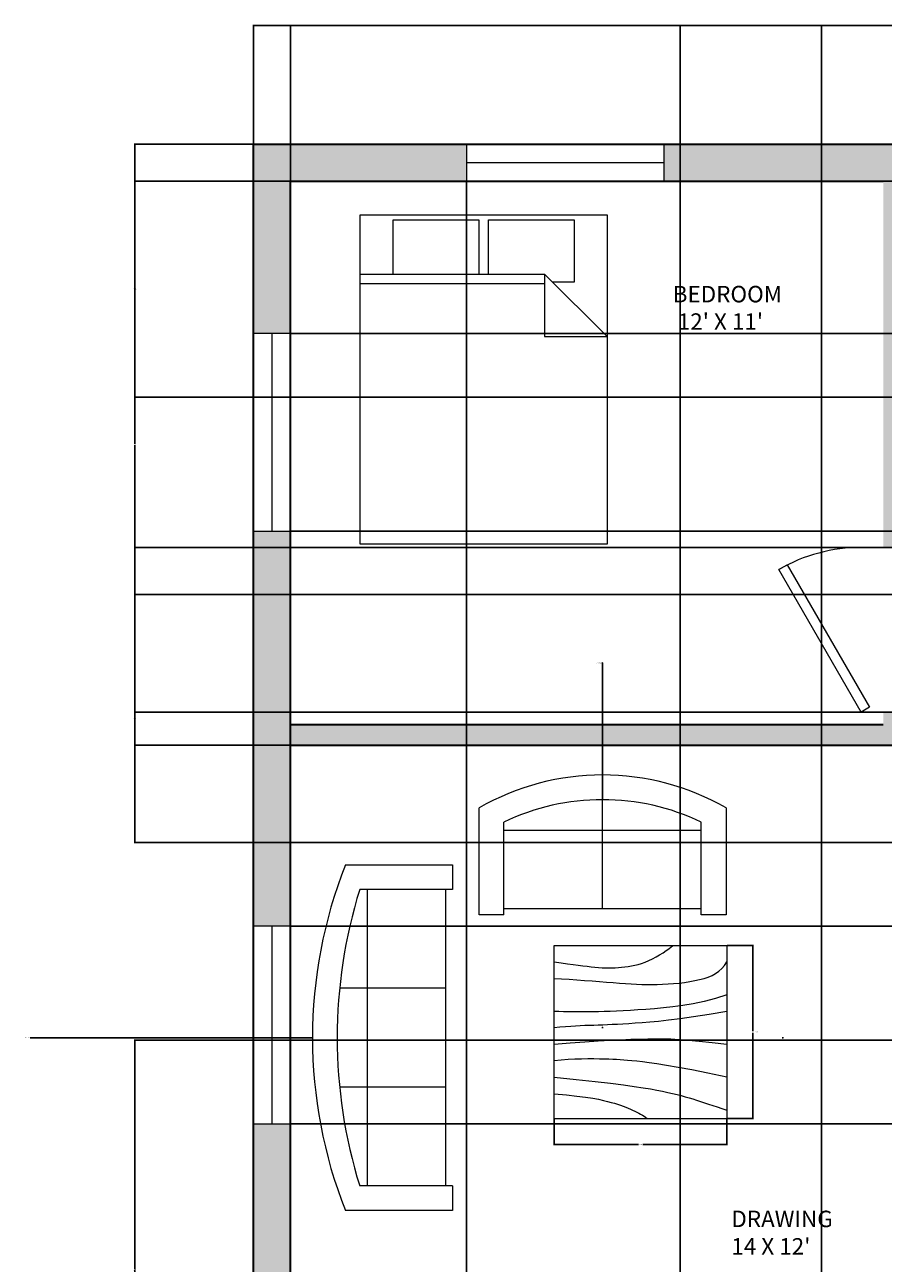
# Model space of a CAD drawing. Units: inches. Extents: x -28 to 649, y -11 to 509.
# Tile 3 of 7: x -28 to 180, y 208 to 509. Entities that reach past the tile are written whole.
import ezdxf

# ---------------------------------------------------------------- set-up
doc = ezdxf.new("R2010")
doc.units = ezdxf.units.IN
doc.header["$MEASUREMENT"] = 0
for name, color, linetype, lineweight in [('A-ANNO-DIMS', 2, 'Continuous', 18), ('A-AREA-IDEN', 18, 'Continuous', 18), ('A-WALL', 7, 'Continuous', 35), ('A-WALL-PATT', 251, 'Continuous', 13), ('doors', 40, 'Continuous', 20), ('furniture', 220, 'Continuous', 18), ('window', 30, 'Continuous', 18)]:
    doc.layers.add(name, color=color, linetype=linetype, lineweight=lineweight)
doc.styles.get("Standard").update_dxf_attribs({"font": 'arial.ttf'})
doc.dimstyles.get("Standard").update_dxf_attribs({"dimtxt": 0.18, "dimasz": 0.18, "dimexe": 0.18, "dimexo": 0.0625, "dimgap": 0.09, "dimtad": 0, "dimtih": 1, "dimtoh": 1, "dimdec": 4, "dimzin": 0, "dimdsep": 46, "dimtxsty": 'Standard', "dimcen": 0.09, "dimadec": 0, "dimazin": 0, "dimtfac": 1, "dimtdec": 4, "dimtofl": 0, "dimtmove": 0, "dimatfit": 3, "dimfxl": 1, "dimtolj": 1, "dimtzin": 0, "dimarcsym": 0})

# ---------------------------------------------------------------- blocks, each defined once
blk = doc.blocks.new('*U9')
for p, q in [((0, 0), (0, -100)), ((750, 0), (750, -100))]:
    blk.add_line(p, q)
blk.add_lwpolyline([(0, 0), (649.5, 375), (671.4, 337.1), (21.9, -37.9)], close=True)
blk.add_arc((0, 0), 750, 0, 30)
blk = doc.blocks.new('Table - Square Woodgrain 42 x 42 in.')
blk.add_line((0, -42), (42, -42))
for points in [[(0, -4), (1.704, -4.2172), (3.2358, -4.4188), (4.615, -4.604), (5.8615, -4.7721), (6.9951, -4.9224), (8.0357, -5.0541), (9.0031, -5.1667), (9.9171, -5.2594), (10.7951, -5.3316), (11.6445, -5.3836), (12.4702, -5.4157), (13.277, -5.4283), (14.0698, -5.4217), (14.8535, -5.3964), (15.6331, -5.3526), (16.4133, -5.2908), (17.1986, -5.2103), (17.9913, -5.1062), (18.793, -4.9727), (19.6056, -4.8038), (20.4307, -4.5937), (21.2701, -4.3365), (22.1256, -4.0262), (22.9989, -3.6571), (23.888, -3.2272), (24.7756, -2.7516), (25.6408, -2.2491), (26.4624, -1.7387), (27.2195, -1.2395), (27.891, -0.7703), (28.456, -0.3501), (28.8934, 0.002)], [(0, -42), (0, 0), (42, 0), (42, -42)], [(0, -8), (1.8203, -8.1001), (3.6741, -8.2149), (5.5411, -8.3408), (7.4011, -8.4741), (9.2339, -8.6112), (11.0193, -8.7484), (12.7371, -8.8821), (14.3671, -9.0086), (15.8954, -9.1246), (17.3337, -9.2278), (18.6997, -9.3159), (20.0116, -9.387), (21.2871, -9.4389), (22.5442, -9.4696), (23.8008, -9.477), (25.0749, -9.459), (26.3791, -9.4137), (27.7049, -9.3403), (29.0383, -9.2382), (30.3655, -9.1068), (31.6728, -8.9455), (32.9461, -8.7535), (34.1717, -8.5304), (35.3358, -8.2756), (36.4268, -7.9863), (37.443, -7.6521), (38.3849, -7.2603), (39.253, -6.7986), (40.048, -6.2542), (40.7705, -5.6147), (41.421, -4.8674), (42, -4)], [(42, -12), (39.1784, -12.8621), (36.4519, -13.5654), (33.8246, -14.1294), (31.3004, -14.5731), (28.8832, -14.9161), (26.577, -15.1775), (24.3858, -15.3768), (22.3136, -15.5332), (20.3622, -15.6632), (18.5254, -15.7718), (16.7947, -15.8612), (15.1618, -15.9338), (13.6183, -15.9916), (12.1558, -16.0369), (10.7659, -16.0718), (9.4403, -16.0987), (8.1703, -16.1191), (6.9461, -16.1325), (5.7577, -16.1377), (4.595, -16.1335), (3.4479, -16.1188), (2.3064, -16.0924), (1.1604, -16.0532), (0, -16)], [(42, -16), (37.6529, -16.7365), (33.8802, -17.329), (30.6179, -17.7961), (27.8015, -18.1561), (25.3668, -18.4275), (23.2497, -18.6288), (21.3859, -18.7785), (19.7111, -18.8949), (18.1693, -18.9939), (16.7375, -19.0795), (15.401, -19.1534), (14.1449, -19.217), (12.9544, -19.2717), (11.8148, -19.3191), (10.7113, -19.3606), (9.6291, -19.3976), (8.5534, -19.4323), (7.47, -19.4689), (6.3643, -19.5122), (5.222, -19.5672), (4.0288, -19.6386), (2.7703, -19.7313), (1.4321, -19.8501), (0, -20)], [(0, -24), (3.9243, -23.6805), (7.4766, -23.4138), (10.6891, -23.1954), (13.5943, -23.0205), (16.2247, -22.8847), (18.6125, -22.7832), (20.7903, -22.7116), (22.7903, -22.6651), (24.6563, -22.642), (26.4764, -22.6507), (28.35, -22.7024), (30.3766, -22.8084), (32.6555, -22.98), (35.2861, -23.2283), (38.3678, -23.5645), (42, -24)], [(42, -32), (37.392, -31.017), (33.4585, -30.2231), (30.1291, -29.5949), (27.3334, -29.109), (25.0009, -28.742), (23.0612, -28.4707), (21.4439, -28.2716), (20.0786, -28.1215), (18.8998, -28.0002), (17.8609, -27.9014), (16.9206, -27.8219), (16.0371, -27.7588), (15.1691, -27.709), (14.2748, -27.6693), (13.3128, -27.6368), (12.2415, -27.6083), (11.0295, -27.5824), (9.6867, -27.5643), (8.233, -27.5608), (6.6884, -27.5787), (5.0728, -27.6248), (3.4062, -27.7058), (1.7086, -27.8286), (0, -28)], [(0, -32), (5.4026, -32.5358), (9.9494, -33.019), (13.7424, -33.4553), (16.8834, -33.8505), (19.4743, -34.2106), (21.6171, -34.5413), (23.4136, -34.8486), (24.9657, -35.1382), (26.3614, -35.4156), (27.6332, -35.6841), (28.7995, -35.9467), (29.8788, -36.2064), (30.8897, -36.4661), (31.8507, -36.7288), (32.7802, -36.9973), (33.6968, -37.2747), (34.6175, -37.5635), (35.5531, -37.8651), (36.5128, -38.1805), (37.506, -38.5108), (38.5421, -38.8568), (39.6302, -39.2197), (40.7797, -39.6004), (42, -40)], [(0, -36), (3.0098, -36.2857), (5.5354, -36.5643), (7.6368, -36.8359), (9.374, -37.1009), (10.807, -37.3597), (11.9957, -37.6126), (13.0002, -37.8599), (13.8804, -38.102), (14.6874, -38.3393), (15.4365, -38.5729), (16.1338, -38.8041), (16.7858, -39.0341), (17.3987, -39.264), (17.9787, -39.4952), (18.5322, -39.7288), (19.0655, -39.9662), (19.5832, -40.2081), (20.0842, -40.4544), (20.5657, -40.7046), (21.0249, -40.9581), (21.459, -41.2144), (21.8653, -41.4731), (22.2409, -41.7335), (22.5831, -41.9951)]]:
    blk.add_lwpolyline(points)
blk = doc.blocks.new('Sofa - Roundback 7 ft.')
for p, q in [((-12.00002, -32.4421), (-12.00003, -6.5971)), ((11.99997, -32.4421), (11.99998, -6.5971)), ((-36.000027, -34), (-36.000027, -11.4696)), ((35.99998, -34), (35.99998, -11.4696)), ((-35.999844, -13.3819), (35.9998, -13.3819)), ((-36.000027, -32.4421), (35.99998, -32.4421))]:
    blk.add_line(p, q)
for points in [[(-36.000027, -34), (-42.000027, -34), (-42.000027, -8)], [(41.99998, -8), (41.99998, -34), (35.99998, -34)]]:
    blk.add_lwpolyline(points)
for centre, radius, start, end in [((0, -114.25), 114.25, 68.43141, 111.5686), ((-0.00001, -127.1968), 121.1968, 72.72033, 107.2797)]:
    blk.add_arc(centre, radius, start, end)
blk = doc.blocks.new('Sofa - Roundback Loveseat 5 ft.')
for p, q in [((0, -32.44198), (0, -5.99998)), ((-24, -33.99998), (-24, -11.46958)), ((24.00004, -33.99998), (24.00004, -11.46958)), ((-23.9998, -13.38178), (23.99986, -13.38178)), ((-24, -32.44198), (24.00004, -32.44198))]:
    blk.add_line(p, q)
for points in [[(-24, -33.99998), (-30, -33.99998), (-30, -7.99998)], [(30.00004, -7.99998), (30.00004, -33.99998), (24.00004, -33.99998)]]:
    blk.add_lwpolyline(points)
for centre, radius, start, end in [((0, -60.24998), 60.24998, 60.13715, 119.8628), ((0, -61.38438), 55.38444, 64.32083, 115.6792)]:
    blk.add_arc(centre, radius, start, end)
blk = doc.blocks.new('Bed - Queen')
for p, q in [((0, -80.00003), (0, 0)), ((0, 0), (59.99999, 0)), ((59.99999, 0), (59.99999, -80.00003)), ((7.99999, -1.2), (28.79998, -1.2)), ((7.99999, -14.4), (7.99999, -1.2)), ((28.79998, -1.2), (28.79998, -14.4)), ((31.19999, -1.2), (51.99999, -1.2)), ((31.19999, -14.4), (31.19999, -1.2)), ((51.99999, -1.2), (51.99999, -16.4)), ((0, -14.4), (44.8, -14.4)), ((59.99999, -29.6), (44.8, -14.4)), ((44.8, -14.4), (44.8, -29.6)), ((44.8, -16.8), (0, -16.8)), ((51.99999, -16.4), (46.79936, -16.4)), ((44.8, -29.6), (59.99999, -29.6)), ((59.99999, -80.00003), (0, -80.00003))]:
    blk.add_line(p, q)
blk = doc.blocks.new('WIN-48x9')
for p, q in [((9, 48), (0, 48)), ((0, 48), (0, 0)), ((4.5, 0), (4.5, 48)), ((9, 0), (9, 48)), ((0, 0), (9, 0)), ((0, 0), (4.5, 0))]:
    blk.add_line(p, q)
blk = doc.blocks.new('*D22')
at = {"layer": 'A-ANNO-DIMS', "color": 0, "lineweight": -2, "transparency": 16777216}
for p, q in [((142.54, 285.23), (148.96, 285.23)), ((148.78, 285.05), (148.78, 264.41)), ((148.78, 243.4), (148.78, 264.04)), ((142.54, 243.22), (148.96, 243.22))]:
    blk.add_line(p, q, dxfattribs=at)
at = {"layer": 'A-ANNO-DIMS', "color": 0, "transparency": 16777216}
for points in [[(148.75, 285.05), (148.81, 285.05), (148.78, 285.23)], [(148.75, 243.4), (148.81, 243.4), (148.78, 243.22)]]:
    blk.add_solid(points, dxfattribs=at)
at = {"layer": 'Defpoints', "color": 0, "transparency": 16777216}
for p in [(142.48, 285.23), (148.78, 285.23), (142.48, 243.22)]:
    blk.add_point(p, dxfattribs=at)
at = {"layer": 'A-ANNO-DIMS', "color": 0, "transparency": 16777216, "insert": (148.78, 264.23), "char_height": 0.18, "attachment_point": 5}
blk.add_mtext('\\A1;SQUARE TABLE 42 TYP.', dxfattribs=at)
blk = doc.blocks.new('*D23')
at = {"layer": 'A-ANNO-DIMS', "color": 0, "lineweight": -2, "transparency": 16777216}
for p, q in [((100.48, 243.16), (100.48, 236.74)), ((142.48, 243.16), (142.48, 236.74)), ((100.66, 236.92), (120.95, 236.92)), ((142.3, 236.92), (122.01, 236.92))]:
    blk.add_line(p, q, dxfattribs=at)
at = {"layer": 'A-ANNO-DIMS', "color": 0, "transparency": 16777216}
for points in [[(100.66, 236.95), (100.66, 236.89), (100.48, 236.92)], [(142.3, 236.95), (142.3, 236.89), (142.48, 236.92)]]:
    blk.add_solid(points, dxfattribs=at)
at = {"layer": 'Defpoints', "color": 0, "transparency": 16777216}
for p in [(100.48, 243.22), (142.48, 243.22), (142.48, 236.92)]:
    blk.add_point(p, dxfattribs=at)
at = {"layer": 'A-ANNO-DIMS', "color": 0, "transparency": 16777216, "insert": (121.48, 236.92), "char_height": 0.18, "attachment_point": 5}
blk.add_mtext('\\A1;42 TYP.', dxfattribs=at)
blk = doc.blocks.new('*D30')
at = {"layer": 'A-ANNO-DIMS', "color": 0, "lineweight": -2, "transparency": 16777216}
for p, q in [((27.45, 480), (27.45, 508.92)), ((27.63, 508.74), (315.16, 508.74)), ((603.27, 508.74), (315.74, 508.74)), ((603.45, 480), (603.45, 508.92))]:
    blk.add_line(p, q, dxfattribs=at)
at = {"layer": 'A-ANNO-DIMS', "color": 0, "transparency": 16777216}
for points in [[(27.63, 508.77), (27.63, 508.71), (27.45, 508.74)], [(603.27, 508.77), (603.27, 508.71), (603.45, 508.74)]]:
    blk.add_solid(points, dxfattribs=at)
at = {"layer": 'Defpoints', "color": 0, "transparency": 16777216}
for p in [(603.45, 508.74), (27.45, 479.94), (603.45, 479.94)]:
    blk.add_point(p, dxfattribs=at)
at = {"layer": 'A-ANNO-DIMS', "color": 0, "transparency": 16777216, "insert": (315.45, 508.74), "char_height": 0.18, "attachment_point": 5}
blk.add_mtext('\\A1;576', dxfattribs=at)
blk = doc.blocks.new('*D36')
at = {"layer": 'A-ANNO-DIMS', "color": 0, "lineweight": -2, "transparency": 16777216}
for p, q in [((27.39, 479.94), (-1.53, 479.94)), ((-1.35, 479.76), (-1.35, 407.12)), ((-1.35, 334.12), (-1.35, 406.76)), ((36.39, 333.94), (-1.53, 333.94))]:
    blk.add_line(p, q, dxfattribs=at)
at = {"layer": 'A-ANNO-DIMS', "color": 0, "transparency": 16777216}
for points in [[(-1.38, 479.76), (-1.32, 479.76), (-1.35, 479.94)], [(-1.38, 334.12), (-1.32, 334.12), (-1.35, 333.94)]]:
    blk.add_solid(points, dxfattribs=at)
at = {"layer": 'Defpoints', "color": 0, "transparency": 16777216}
for p in [(-1.35, 479.94), (27.45, 479.94), (36.45, 333.94)]:
    blk.add_point(p, dxfattribs=at)
at = {"layer": 'A-ANNO-DIMS', "color": 0, "transparency": 16777216, "insert": (-1.35, 406.94), "char_height": 0.18, "attachment_point": 5}
blk.add_mtext('\\A1;146', dxfattribs=at)
blk = doc.blocks.new('*D44')
at = {"layer": 'A-ANNO-DIMS', "color": 0, "lineweight": -2, "transparency": 16777216}
for p, q in [((36.45, 470.88), (36.45, -11.04)), ((79.22, 470.88), (79.22, -11.04)), ((36.63, -10.86), (57.44, -10.86)), ((79.04, -10.86), (58.23, -10.86))]:
    blk.add_line(p, q, dxfattribs=at)
at = {"layer": 'A-ANNO-DIMS', "color": 0, "transparency": 16777216}
for points in [[(36.63, -10.83), (36.63, -10.89), (36.45, -10.86)], [(79.04, -10.83), (79.04, -10.89), (79.22, -10.86)]]:
    blk.add_solid(points, dxfattribs=at)
at = {"layer": 'Defpoints', "color": 0, "transparency": 16777216}
for p in [(36.45, 470.94), (79.22, 470.94), (79.22, -10.86)]:
    blk.add_point(p, dxfattribs=at)
at = {"layer": 'A-ANNO-DIMS', "color": 0, "transparency": 16777216, "insert": (57.83, -10.86), "char_height": 0.18, "attachment_point": 5}
blk.add_mtext('\\A1;42.77', dxfattribs=at)
blk = doc.blocks.new('*D49')
at = {"layer": 'A-ANNO-DIMS', "color": 0, "lineweight": -2, "transparency": 16777216}
for p, q in [((36.51, 470.94), (632.43, 470.94)), ((632.25, 470.76), (632.25, 452.59)), ((632.25, 434.06), (632.25, 452.23)), ((36.51, 433.88), (632.43, 433.88))]:
    blk.add_line(p, q, dxfattribs=at)
at = {"layer": 'A-ANNO-DIMS', "color": 0, "transparency": 16777216}
for points in [[(632.22, 470.76), (632.28, 470.76), (632.25, 470.94)], [(632.22, 434.06), (632.28, 434.06), (632.25, 433.88)]]:
    blk.add_solid(points, dxfattribs=at)
at = {"layer": 'Defpoints', "color": 0, "transparency": 16777216}
for p in [(36.45, 470.94), (36.45, 433.88), (632.25, 433.88)]:
    blk.add_point(p, dxfattribs=at)
at = {"layer": 'A-ANNO-DIMS', "color": 0, "transparency": 16777216, "insert": (632.25, 452.41), "char_height": 0.18, "attachment_point": 5}
blk.add_mtext('\\A1;37.055', dxfattribs=at)
blk = doc.blocks.new('*D50')
at = {"layer": 'A-ANNO-DIMS', "color": 0, "lineweight": -2, "transparency": 16777216}
for p, q in [((594.39, 470.94), (-1.53, 470.94)), ((-1.35, 470.76), (-1.35, 444.89)), ((-1.35, 418.66), (-1.35, 444.53)), ((594.39, 418.48), (-1.53, 418.48))]:
    blk.add_line(p, q, dxfattribs=at)
at = {"layer": 'A-ANNO-DIMS', "color": 0, "transparency": 16777216}
for points in [[(-1.38, 470.76), (-1.32, 470.76), (-1.35, 470.94)], [(-1.38, 418.66), (-1.32, 418.66), (-1.35, 418.48)]]:
    blk.add_solid(points, dxfattribs=at)
at = {"layer": 'Defpoints', "color": 0, "transparency": 16777216}
for p in [(594.45, 470.94), (-1.35, 418.48), (594.45, 418.48)]:
    blk.add_point(p, dxfattribs=at)
at = {"layer": 'A-ANNO-DIMS', "color": 0, "transparency": 16777216, "insert": (-1.35, 444.71), "char_height": 0.18, "attachment_point": 5}
blk.add_mtext('\\A1;52.46', dxfattribs=at)
blk = doc.blocks.new('*D51')
at = {"layer": 'A-ANNO-DIMS', "color": 0, "lineweight": -2, "transparency": 16777216}
for p, q in [((594.39, 370.48), (-1.53, 370.48)), ((-1.35, 370.3), (-1.35, 340.55)), ((-1.35, 310.43), (-1.35, 340.19)), ((594.39, 310.25), (-1.53, 310.25))]:
    blk.add_line(p, q, dxfattribs=at)
at = {"layer": 'A-ANNO-DIMS', "color": 0, "transparency": 16777216}
for points in [[(-1.38, 370.3), (-1.32, 370.3), (-1.35, 370.48)], [(-1.38, 310.43), (-1.32, 310.43), (-1.35, 310.25)]]:
    blk.add_solid(points, dxfattribs=at)
at = {"layer": 'Defpoints', "color": 0, "transparency": 16777216}
for p in [(-1.35, 370.48), (594.45, 370.48), (594.45, 310.25)]:
    blk.add_point(p, dxfattribs=at)
at = {"layer": 'A-ANNO-DIMS', "color": 0, "transparency": 16777216, "insert": (-1.35, 340.37), "char_height": 0.18, "attachment_point": 5}
blk.add_mtext('\\A1;60.23', dxfattribs=at)
blk = doc.blocks.new('*D52')
at = {"layer": 'A-ANNO-DIMS', "color": 0, "lineweight": -2, "transparency": 16777216}
for p, q in [((594.39, 262.25), (-1.53, 262.25)), ((-1.35, 262.07), (-1.35, 206.61)), ((-1.35, 150.79), (-1.35, 206.25)), ((594.39, 150.61), (-1.53, 150.61))]:
    blk.add_line(p, q, dxfattribs=at)
at = {"layer": 'A-ANNO-DIMS', "color": 0, "transparency": 16777216}
for points in [[(-1.38, 262.07), (-1.32, 262.07), (-1.35, 262.25)], [(-1.38, 150.79), (-1.32, 150.79), (-1.35, 150.61)]]:
    blk.add_solid(points, dxfattribs=at)
at = {"layer": 'Defpoints', "color": 0, "transparency": 16777216}
for p in [(-1.35, 262.25), (594.45, 262.25), (594.45, 150.61)]:
    blk.add_point(p, dxfattribs=at)
at = {"layer": 'A-ANNO-DIMS', "color": 0, "transparency": 16777216, "insert": (-1.35, 206.43), "char_height": 0.18, "attachment_point": 5}
blk.add_mtext('\\A1;111.64', dxfattribs=at)
blk = doc.blocks.new('*D53')
at = {"layer": 'A-ANNO-DIMS', "color": 0, "lineweight": -2, "transparency": 16777216}
for p, q in [((36.51, 241.9), (632.43, 241.9)), ((632.25, 241.72), (632.25, 191.76)), ((632.25, 141.44), (632.25, 191.39)), ((36.51, 141.26), (632.43, 141.26))]:
    blk.add_line(p, q, dxfattribs=at)
at = {"layer": 'A-ANNO-DIMS', "color": 0, "transparency": 16777216}
for points in [[(632.22, 241.72), (632.28, 241.72), (632.25, 241.9)], [(632.22, 141.44), (632.28, 141.44), (632.25, 141.26)]]:
    blk.add_solid(points, dxfattribs=at)
at = {"layer": 'Defpoints', "color": 0, "transparency": 16777216}
for p in [(36.45, 241.9), (632.25, 241.9), (36.45, 141.26)]:
    blk.add_point(p, dxfattribs=at)
at = {"layer": 'A-ANNO-DIMS', "color": 0, "transparency": 16777216, "insert": (632.25, 191.58), "char_height": 0.18, "attachment_point": 5}
blk.add_mtext('\\A1;100.64', dxfattribs=at)
blk = doc.blocks.new('*D54')
at = {"layer": 'A-ANNO-DIMS', "color": 0, "lineweight": -2, "transparency": 16777216}
for p, q in [((36.51, 385.88), (632.43, 385.88)), ((632.25, 385.7), (632.25, 338.07)), ((632.25, 290.08), (632.25, 337.71)), ((36.51, 289.9), (632.43, 289.9))]:
    blk.add_line(p, q, dxfattribs=at)
at = {"layer": 'A-ANNO-DIMS', "color": 0, "transparency": 16777216}
for points in [[(632.22, 385.7), (632.28, 385.7), (632.25, 385.88)], [(632.22, 290.08), (632.28, 290.08), (632.25, 289.9)]]:
    blk.add_solid(points, dxfattribs=at)
at = {"layer": 'Defpoints', "color": 0, "transparency": 16777216}
for p in [(36.45, 385.88), (632.25, 385.88), (36.45, 289.9)]:
    blk.add_point(p, dxfattribs=at)
at = {"layer": 'A-ANNO-DIMS', "color": 0, "transparency": 16777216, "insert": (632.25, 337.89), "char_height": 0.18, "attachment_point": 5}
blk.add_mtext('\\A1;95.99', dxfattribs=at)
blk = doc.blocks.new('*D55')
at = {"layer": 'A-ANNO-DIMS', "color": 0, "lineweight": -2, "transparency": 16777216}
for p, q in [((36.45, 57), (36.45, 508.92)), ((36.63, 508.74), (83.39, 508.74)), ((130.94, 508.74), (84.18, 508.74)), ((131.12, 57), (131.12, 508.92))]:
    blk.add_line(p, q, dxfattribs=at)
at = {"layer": 'A-ANNO-DIMS', "color": 0, "transparency": 16777216}
for points in [[(36.63, 508.77), (36.63, 508.71), (36.45, 508.74)], [(130.94, 508.77), (130.94, 508.71), (131.12, 508.74)]]:
    blk.add_solid(points, dxfattribs=at)
at = {"layer": 'Defpoints', "color": 0, "transparency": 16777216}
for p in [(131.12, 508.74), (36.45, 56.94), (131.12, 56.94)]:
    blk.add_point(p, dxfattribs=at)
at = {"layer": 'A-ANNO-DIMS', "color": 0, "transparency": 16777216, "insert": (83.79, 508.74), "char_height": 0.18, "attachment_point": 5}
blk.add_mtext('\\A1;94.67', dxfattribs=at)
blk = doc.blocks.new('*D57')
at = {"layer": 'A-ANNO-DIMS', "color": 0, "lineweight": -2, "transparency": 16777216}
for p, q in [((165.45, 190), (165.45, 508.92)), ((165.63, 508.74), (183.23, 508.74)), ((201.27, 508.74), (183.67, 508.74)), ((201.45, 190), (201.45, 508.92))]:
    blk.add_line(p, q, dxfattribs=at)
at = {"layer": 'A-ANNO-DIMS', "color": 0, "transparency": 16777216}
for points in [[(165.63, 508.77), (165.63, 508.71), (165.45, 508.74)], [(201.27, 508.77), (201.27, 508.71), (201.45, 508.74)]]:
    blk.add_solid(points, dxfattribs=at)
at = {"layer": 'Defpoints', "color": 0, "transparency": 16777216}
for p in [(201.45, 508.74), (165.45, 189.94), (201.45, 189.94)]:
    blk.add_point(p, dxfattribs=at)
at = {"layer": 'A-ANNO-DIMS', "color": 0, "transparency": 16777216, "insert": (183.45, 508.74), "char_height": 0.18, "attachment_point": 5}
blk.add_mtext('\\A1;36', dxfattribs=at)
blk = doc.blocks.new('*D66')
at = {"layer": 'A-ANNO-DIMS', "color": 0, "lineweight": -2, "transparency": 16777216}
for p, q in [((447.05, 381.94), (-1.53, 381.94)), ((-1.35, 381.76), (-1.35, 362.12)), ((-1.35, 342.12), (-1.35, 361.76)), ((447.39, 341.94), (-1.53, 341.94))]:
    blk.add_line(p, q, dxfattribs=at)
at = {"layer": 'A-ANNO-DIMS', "color": 0, "transparency": 16777216}
for points in [[(-1.38, 381.76), (-1.32, 381.76), (-1.35, 381.94)], [(-1.38, 342.12), (-1.32, 342.12), (-1.35, 341.94)]]:
    blk.add_solid(points, dxfattribs=at)
at = {"layer": 'Defpoints', "color": 0, "transparency": 16777216}
for p in [(-1.35, 381.94), (447.12, 381.94), (447.45, 341.94)]:
    blk.add_point(p, dxfattribs=at)
at = {"layer": 'A-ANNO-DIMS', "color": 0, "transparency": 16777216, "insert": (-1.35, 361.94), "char_height": 0.18, "attachment_point": 5}
blk.add_mtext('\\A1;40', dxfattribs=at)
blk = doc.blocks.new('*D78')
at = {"layer": 'A-ANNO-DIMS', "color": 0, "lineweight": -2, "transparency": 16777216}
for p, q in [((-26.78, 262.83), (41.59, 262.83)), ((155.93, 262.83), (156.11, 262.83)), ((156.02, 262.74), (156.02, 262.92))]:
    blk.add_line(p, q, dxfattribs=at)
at = {"layer": 'A-ANNO-DIMS', "color": 0, "transparency": 16777216}
blk.add_solid([(41.59, 262.86), (41.59, 262.8), (41.77, 262.83)], dxfattribs=at)
at = {"layer": 'Defpoints', "color": 0, "transparency": 16777216}
for p in [(41.77, 262.83), (156.02, 262.83)]:
    blk.add_point(p, dxfattribs=at)
at = {"layer": 'A-ANNO-DIMS', "color": 0, "transparency": 16777216, "insert": (-27.52, 262.83), "char_height": 0.18, "attachment_point": 5}
blk.add_mtext('\\A1;2X R114.25', dxfattribs=at)
blk = doc.blocks.new('*D80')
at = {"layer": 'A-ANNO-DIMS', "color": 0, "lineweight": -2, "transparency": 16777216}
for p, q in [((112.07, 353.89), (112.25, 353.89)), ((112.25, 353.89), (112.25, 320.84)), ((112.16, 265.27), (112.34, 265.27)), ((112.25, 265.18), (112.25, 265.36))]:
    blk.add_line(p, q, dxfattribs=at)
at = {"layer": 'A-ANNO-DIMS', "color": 0, "transparency": 16777216}
blk.add_solid([(112.28, 320.84), (112.22, 320.84), (112.25, 320.66)], dxfattribs=at)
at = {"layer": 'Defpoints', "color": 0, "transparency": 16777216}
for p in [(112.25, 320.66), (112.25, 265.27)]:
    blk.add_point(p, dxfattribs=at)
at = {"layer": 'A-ANNO-DIMS', "color": 0, "transparency": 16777216, "insert": (111.39, 353.89), "char_height": 0.18, "attachment_point": 5}
blk.add_mtext('\\A1;2X R55.38', dxfattribs=at)

msp = doc.modelspace()

# ---------------------------------------------------------------- hatches: boundary and pattern name
at = {"layer": 'A-WALL-PATT'}
h = msp.add_hatch(color=256, dxfattribs=at)
h.dxf.hatch_style = 1
h.paths.add_polyline_path([(36.4499, 184.9382), (165.4499, 184.9382), (165.4499, 189.9382), (36.4499, 189.9382), (36.4499, 241.898), (27.4499, 241.898), (27.4499, 141.2558), (36.4499, 141.2558)])
h.paths.add_polyline_path([(36.4499, 385.8835), (27.4499, 385.8835), (27.4499, 289.898), (36.4499, 289.898)])
h.paths.add_polyline_path([(185.4499, 341.9382), (180.4499, 341.9382), (180.4499, 338.9382), (36.4499, 338.9382), (36.4499, 333.9382), (185.4499, 333.9382)])
h.paths.add_polyline_path([(36.4499, 470.9382), (79.2168, 470.9382), (79.2168, 479.9382), (27.4499, 479.9382), (27.4499, 433.8835), (36.4499, 433.8835)])
h.paths.add_polyline_path([(185.4499, 470.9382), (203.9104, 470.9382), (203.9104, 479.9382), (127.2168, 479.9382), (127.2168, 470.9382), (180.4499, 470.9382), (180.4499, 381.9382), (188.4499, 381.9382), (188.4499, 386.9382), (185.4499, 386.9382)])
h.paths.add_polyline_path([(292.4601, 479.9382), (227.9104, 479.9382), (227.9104, 470.9382), (245.4499, 470.9382), (245.4499, 386.9382), (217.4499, 386.9382), (217.4499, 381.9382), (245.4499, 381.9382), (245.4499, 338.9382), (245.4499, 333.9382), (251.5222, 333.9382), (251.5222, 338.9382), (250.4499, 338.9382), (250.4499, 470.9382), (292.4601, 470.9382)])
h.paths.add_polyline_path([(410.9121, 479.9382), (340.4601, 479.9382), (340.4601, 470.9382), (382.4499, 470.9382), (382.4499, 338.9382), (287.5222, 338.9382), (287.5222, 333.9382), (387.4499, 333.9382), (387.4499, 381.9382), (415.4499, 381.9382), (415.4499, 386.9382), (387.4499, 386.9382), (387.4499, 470.9382), (410.9121, 470.9382)])
h.paths.add_polyline_path([(497.0961, 479.9382), (434.9121, 479.9382), (434.9121, 470.9382), (447.4499, 470.9382), (447.4499, 386.9382), (444.4499, 386.9382), (444.4499, 381.9382), (452.4499, 381.9382), (452.4499, 470.9382), (497.0961, 470.9382)])
h.paths.add_polyline_path([(603.4499, 479.9382), (545.0961, 479.9382), (545.0961, 470.9382), (594.4499, 470.9382), (594.4499, 418.4819), (603.4499, 418.4819)])
h.paths.add_polyline_path([(603.4499, 370.4819), (594.4499, 370.4819), (594.4499, 338.9382), (452.4499, 338.9382), (452.4499, 341.9382), (447.4499, 341.9382), (447.4499, 338.9382), (447.4499, 333.9382), (594.4499, 333.9382), (594.4499, 310.2528), (603.4499, 310.2528)])
h.paths.add_polyline_path([(603.4499, 262.2528), (594.4499, 262.2528), (594.4499, 205.9382), (515.4499, 205.9382), (515.4499, 200.9382), (594.4499, 200.9382), (594.4499, 150.6102), (603.4499, 150.6102)])

# ---------------------------------------------------------------- linework, layer by layer
at = {"layer": 'A-WALL'}
for p, q in [((36.4499, 470.9382), (180.4499, 470.9382)), ((36.4499, 189.9382), (36.4499, 470.9382)), ((36.4499, 338.9382), (180.4499, 338.9382)), ((36.4499, 333.9382), (185.4499, 333.9382))]:
    msp.add_line(p, q, dxfattribs=at)
msp.add_lwpolyline([(209.4499, 47.9382), (27.4499, 47.9382), (27.4499, 479.9382), (603.4499, 479.9382), (603.4499, 47.9382), (269.4499, 47.9382)], dxfattribs=at)

# ---------------------------------------------------------------- block references
at = {"layer": 'doors', "xscale": 0.0533333333333332, "yscale": 0.0533333333333332, "zscale": 0.0533333333333332, "rotation": 90}
msp.add_blockref('*U9', (175.1165, 341.9382), dxfattribs=at)
at = {"layer": 'furniture'}
for name, p in [('Bed - Queen', (53.3555, 462.7454)), ('Sofa - Roundback Loveseat 5 ft.', (112.2492, 326.6552)), ('Table - Square Woodgrain 42 x 42 in.', (100.4781, 285.2247))]:
    msp.add_blockref(name, p, dxfattribs=at)
at = {"layer": 'furniture', "rotation": 90}
msp.add_blockref('Sofa - Roundback 7 ft.', (41.7732, 262.8262), dxfattribs=at)
at = {"layer": 'window', "rotation": 269.9999999999889}
msp.add_blockref('WIN-48x9', (79.2168, 479.9382), dxfattribs=at)
at = {"layer": 'window'}
for p in [(27.4499, 385.8835), (27.4499, 241.898)]:
    msp.add_blockref('WIN-48x9', p, dxfattribs=at)

# ---------------------------------------------------------------- texts
at = {"layer": 'A-AREA-IDEN', "char_height": 4, "attachment_point": 1}
for s, insert in [("BEDROOM\\P 12' X 11'", (129.3084, 445.4773)), (" DRAWING\\P 14 X 12'", (142.3287, 220.8043))]:
    msp.add_mtext_dynamic_manual_height_columns(s, width=46.696275, gutter_width=1, heights=[0], dxfattribs=dict(at, insert=insert))

# ---------------------------------------------------------------- dimensions: what is measured, and where the dimension line sits
at = {"layer": 'A-ANNO-DIMS'}
for base, p1, p2, override, picture, middle in [((603.4499, 508.7392), (27.4499, 479.9382), (603.4499, 479.9382), {"dimdec": 0, "dimlfac": 1, "dimrnd": 0, "dimzin": 0, "dimdsep": 46, "dimlunit": 2}, '*D30', (315.4499, 508.7392)), ((131.1226, 508.7392), (36.4499, 56.9382), (131.1226, 56.9382), {"dimdec": 2, "dimlfac": 1, "dimrnd": 0, "dimzin": 0, "dimdsep": 46, "dimlunit": 2}, '*D55', (83.7862, 508.7392)), ((201.4499, 508.7392), (165.4499, 189.9382), (201.4499, 189.9382), {"dimdec": 0, "dimlfac": 1, "dimrnd": 0, "dimzin": 0, "dimdsep": 46, "dimlunit": 2}, '*D57', (183.4499, 508.7392)), ((79.2168, -10.8628), (36.4499, 470.9382), (79.2168, 470.9382), {"dimdec": 2, "dimlfac": 1, "dimrnd": 0, "dimzin": 0, "dimdsep": 46, "dimlunit": 2}, '*D44', (57.8333, -10.8628))]:
    dim = msp.add_linear_dim(base=base, p1=p1, p2=p2, dimstyle='Standard', override=override, dxfattribs=at)
    dim.commit()
    dim.dimension.update_dxf_attribs({"geometry": picture, "text_midpoint": middle})
for base, p1, p2, override, picture, middle in [((-1.3511, 479.9382), (36.4499, 333.9382), (27.4499, 479.9382), {"dimdec": 0, "dimlfac": 1, "dimrnd": 0, "dimzin": 0, "dimdsep": 46, "dimlunit": 2}, '*D36', (-1.3511, 406.9382)), ((-1.3511, 418.4819), (594.4499, 470.9382), (594.4499, 418.4819), {"dimdec": 2, "dimlfac": 1, "dimrnd": 0, "dimzin": 0, "dimdsep": 46, "dimlunit": 2}, '*D50', (-1.3511, 444.71)), ((632.2509, 433.8835), (36.4499, 470.9382), (36.4499, 433.8835), {"dimdec": 3, "dimlfac": 1, "dimrnd": 0, "dimzin": 0, "dimdsep": 46, "dimlunit": 2}, '*D49', (632.2509, 452.4109)), ((632.2509, 385.8835), (36.4499, 289.898), (36.4499, 385.8835), {"dimdec": 2, "dimlfac": 1, "dimrnd": 0, "dimzin": 0, "dimdsep": 46, "dimlunit": 2}, '*D54', (632.2509, 337.8907)), ((-1.3511, 381.9382), (447.4499, 341.9382), (447.1165, 381.9382), {"dimdec": 0, "dimlfac": 1, "dimrnd": 0, "dimzin": 0, "dimdsep": 46, "dimlunit": 2}, '*D66', (-1.3511, 361.9382)), ((-1.3511, 370.4819), (594.4499, 310.2528), (594.4499, 370.4819), {"dimdec": 2, "dimlfac": 1, "dimrnd": 0, "dimzin": 0, "dimdsep": 46, "dimlunit": 2}, '*D51', (-1.3511, 340.3674)), ((-1.3511, 262.2528), (594.4499, 150.6102), (594.4499, 262.2528), {"dimdec": 2, "dimlfac": 1, "dimrnd": 0, "dimzin": 0, "dimdsep": 46, "dimlunit": 2}, '*D52', (-1.3511, 206.4315)), ((632.2509, 241.898), (36.4499, 141.2558), (36.4499, 241.898), {"dimdec": 2, "dimlfac": 1, "dimrnd": 0, "dimzin": 0, "dimdsep": 46, "dimlunit": 2}, '*D53', (632.2509, 191.5769))]:
    dim = msp.add_linear_dim(base=base, p1=p1, p2=p2, angle=90, dimstyle='Standard', override=override, dxfattribs=at)
    dim.commit()
    dim.dimension.update_dxf_attribs({"geometry": picture, "text_midpoint": middle})
for center, mpoint, picture, middle in [((112.2492, 265.2708), (112.249, 320.6552), '*D80', (111.394, 353.8859)), ((156.0232, 262.8262), (41.7732, 262.826), '*D78', (-26.7768, 262.8259))]:
    dim = msp.add_radius_dim(center=center, mpoint=mpoint, text='2X <>', dimstyle='Standard', override={"dimdec": 2, "dimlfac": 1, "dimrnd": 0, "dimzin": 0, "dimdsep": 46, "dimlunit": 2}, dxfattribs=at)
    dim.commit()
    dim.dimension.update_dxf_attribs({"geometry": picture, "text_midpoint": middle, "dimtype": 164})
dim = msp.add_linear_dim(base=(148.7784, 285.2267), p1=(142.4781, 243.2247), p2=(142.4781, 285.2267), angle=90, text='SQUARE TABLE <> TYP.', dimstyle='Standard', override={"dimdec": 0, "dimlfac": 1, "dimrnd": 0, "dimzin": 0, "dimdsep": 46, "dimlunit": 2}, dxfattribs=at)
dim.commit()
dim.dimension.update_dxf_attribs({"geometry": '*D22', "text_midpoint": (148.7784, 264.2257)})
dim = msp.add_linear_dim(base=(142.4781, 236.9244), p1=(100.4781, 243.2247), p2=(142.4781, 243.2247), text='<> TYP.', dimstyle='Standard', override={"dimdec": 0, "dimlfac": 1, "dimrnd": 0, "dimzin": 0, "dimdsep": 46, "dimlunit": 2}, dxfattribs=at)
dim.commit()
dim.dimension.update_dxf_attribs({"geometry": '*D23', "text_midpoint": (121.4781, 236.9244)})

doc.saveas('drawing.dxf')
